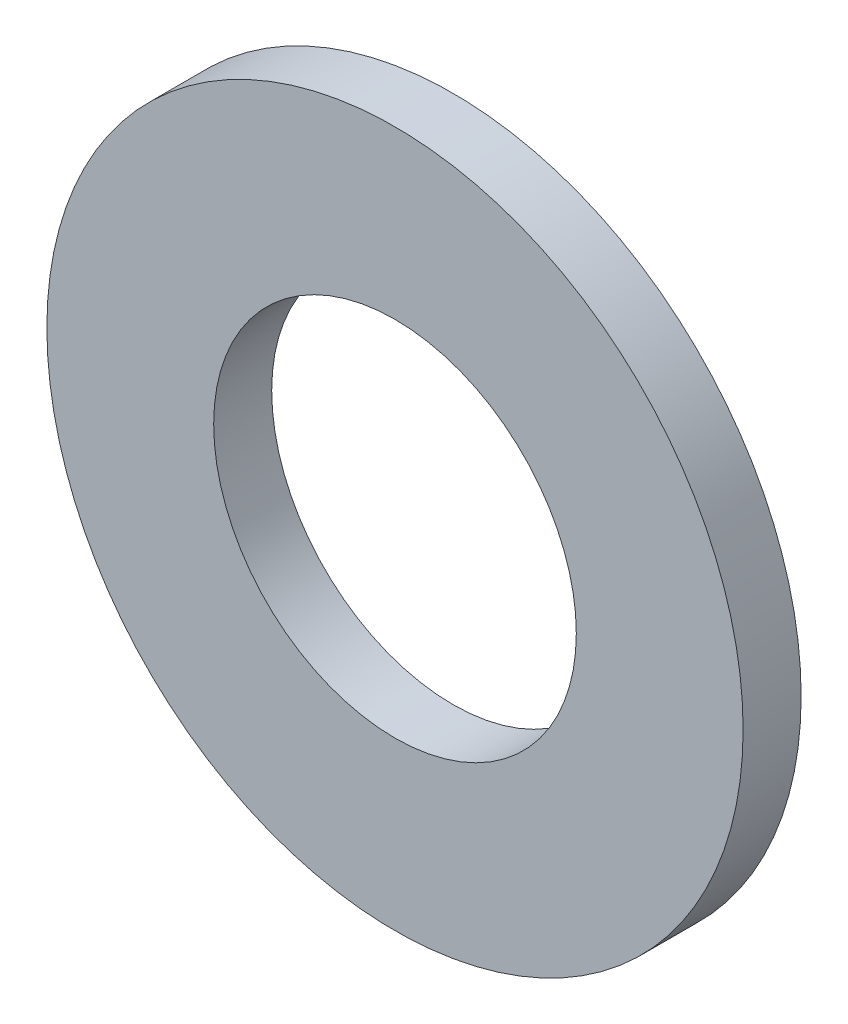
from build123d import *

# Parameters (mm, degrees)
WASHER_PROFILE_12_X_6_25_R   = 6
WASHER_PROFILE_12_X_6_25_R_2 = 3.125
WASHER_BODY_1MM_DEPTH        = 0.5


with BuildPart() as part:
    # Washer Profile Ø12 x Ø6.25 → Washer Body 1mm (new, symmetric)
    with BuildSketch(Plane.XY):
        Circle(WASHER_PROFILE_12_X_6_25_R)
        Circle(WASHER_PROFILE_12_X_6_25_R_2, mode=Mode.SUBTRACT)
    extrude(amount=WASHER_BODY_1MM_DEPTH, both=True)


solid = part.part
